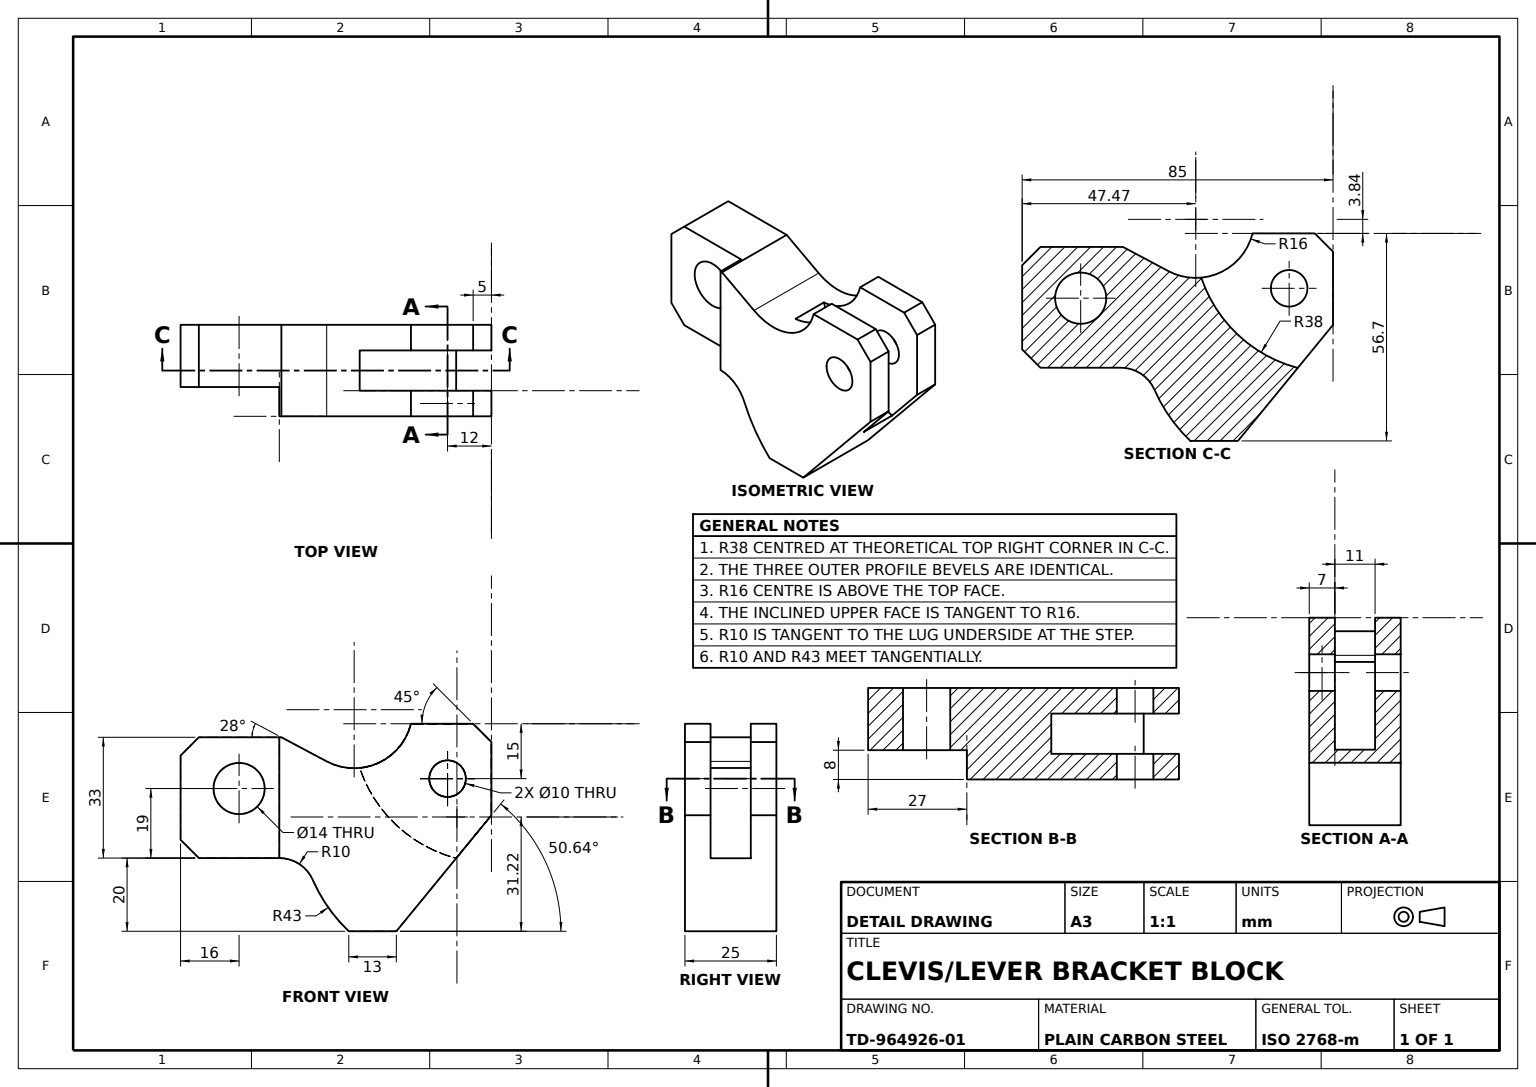
from build123d import *

# Parameters (mm, degrees)
BRACKET_PROFILE_SKETCH_R   = 5
BRACKET_PROFILE_SKETCH_R_2 = 7
BRACKET_BODY_25MM_DEPTH    = 12.5
FORK_SLOT_SKETCH_W         = 27
FORK_SLOT_SKETCH_H         = 8
FORK_SLOT_8X27_DEPTH       = 63
RELIEF_CIRCLE_SKETCH_76_R  = 38
FRONT_RELIEF_CUT_76_DEPTH  = 5.5


with BuildPart() as part:
    # Bracket Profile Sketch → Bracket Body 25mm (new, symmetric)
    with BuildSketch(Plane.XY):
        with BuildLine():
            Line((-1.467633793, -60.539351202), (11.532366207, -60.539351202))
            Line((11.532366207, -60.539351202), (37.532366207, -28.84))
            Line((37.532366207, -28.84), (37.532366207, -8.84))
            Line((37.532366207, -8.84), (32.532366207, -3.84))
            Line((32.532366207, -3.84), (15.532366207, -3.84))
            ThreePointArc((15.532366207, -3.84), (6.522255442, -14.610276655), (-7.511545005, -14.127161486))
            Line((-7.511545005, -14.127161486), (-19.901414154, -7.539351202))
            Line((-19.901414154, -7.539351202), (-42.467633793, -7.539351202))
            Line((-42.467633793, -7.539351202), (-47.467633793, -12.539351202))
            Line((-47.467633793, -12.539351202), (-47.467633793, -35.539351202))
            Line((-47.467633793, -35.539351202), (-42.467633793, -40.539351202))
            Line((-42.467633793, -40.539351202), (-20.467867574, -40.539351202))
            ThreePointArc((-20.467867574, -40.539351202), (-14.992702243, -42.171402553), (-11.304687106, -46.534838282))
            ThreePointArc((-11.304687106, -46.534838282), (-7.089928905, -54.031435949), (-1.467633793, -60.539351202))
        make_face()
        with Locations((25.532366207, -18.84)):
            Circle(BRACKET_PROFILE_SKETCH_R, mode=Mode.SUBTRACT)
        with Locations((-31.467633793, -21.539351202)):
            Circle(BRACKET_PROFILE_SKETCH_R_2, mode=Mode.SUBTRACT)
    extrude(amount=BRACKET_BODY_25MM_DEPTH, both=True)

    # Fork Slot Sketch → Fork Slot 8x27 (cut)
    with BuildSketch(Plane(origin=(0, 0, 0), x_dir=(1, 0, 0), z_dir=(0, 1, 0))):
        with Locations((-33.967633793, -8.5)):
            Rectangle(FORK_SLOT_SKETCH_W, FORK_SLOT_SKETCH_H)
    extrude(amount=-FORK_SLOT_8X27_DEPTH, mode=Mode.SUBTRACT)

    # Relief Circle Sketch Ø76 → Front Relief Cut Ø76 (cut, symmetric)
    with BuildSketch(Plane.XY):
        with Locations((37.532366207, -3.84)):
            Circle(RELIEF_CIRCLE_SKETCH_76_R)
    extrude(amount=FRONT_RELIEF_CUT_76_DEPTH, both=True, mode=Mode.SUBTRACT)


solid = part.part
